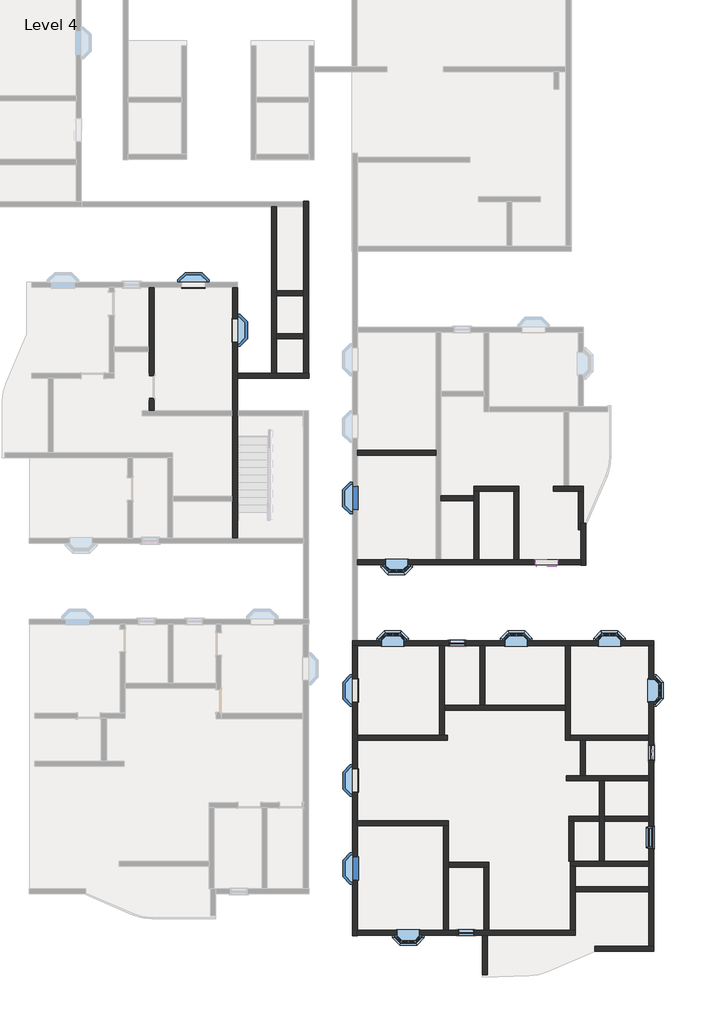
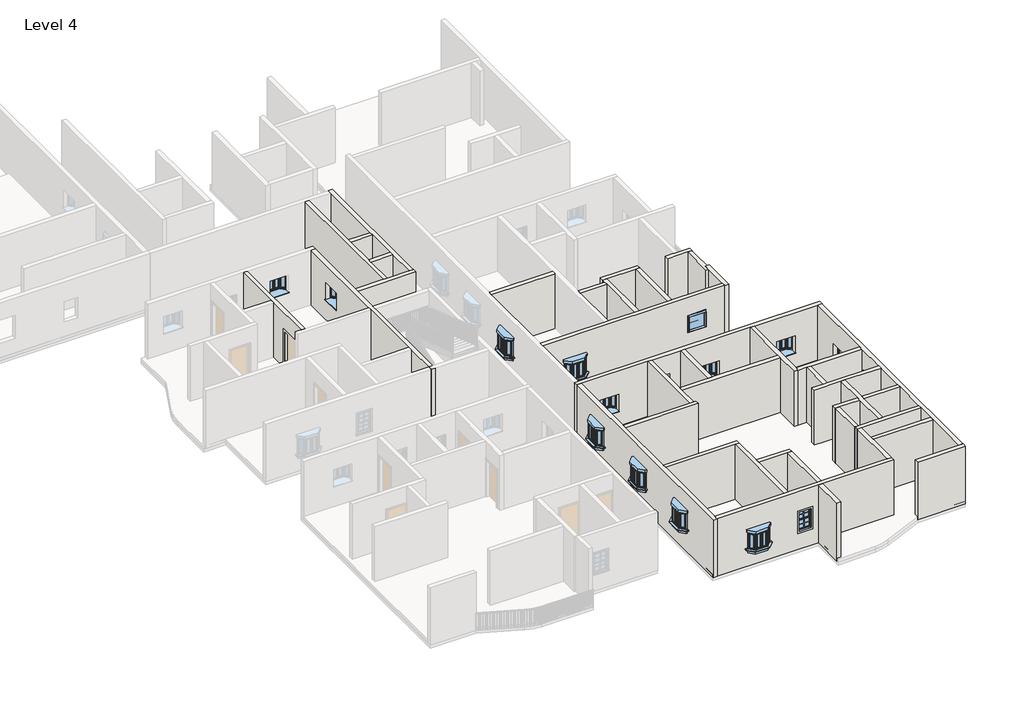
# One storey, part 2 of 14: 40 walls, 17 windows.
# Revit data of these elements (continued)
# Element 46 (IfcWindow, "910x910mm") (continued)
#   Materials on its faces: "Window Frame", "Glass"
# Element 47 (IfcWindow, "910x910mm")
#   Mark = "190"
#   Phase Created = New Construction
#   Materials on its faces: "Window Frame", "Glass"
# Element 48 (IfcWindow, "910x910mm")
#   Mark = "191"
#   Phase Created = New Construction
#   Materials on its faces: "Window Frame", "Glass"
# Element 49 (IfcWindow, "910x910mm")
#   Mark = "192"
#   Phase Created = New Construction
#   Materials on its faces: "Window Frame", "Glass"
# Element 50 (IfcWindow, "910x910mm")
#   Mark = "193"
#   Phase Created = New Construction
#   Materials on its faces: "Window Frame", "Glass"
# Element 51 (IfcWindow, "910x910mm")
#   Mark = "194"
#   Phase Created = New Construction
#   Materials on its faces: "Window Frame", "Glass"
# Element 52 (IfcWindow, "910x910mm")
#   Mark = "195"
#   Phase Created = New Construction
#   Materials on its faces: "Window Frame", "Glass"
# Element 53 (IfcWindow, "Window-Double-Hung : 26\" x 42\"")
#   Mark = "218"
#   Window Inset = 0' - 0"
#   Interior Wall Closure = 0' - 1 1/2"
#   Frame Extension = 0' - 1 1/4"
#   Exterior Wall Closure = 0' - 0 1/2"
#   Interior Trim Visibility = yes
#   Indicator Visibility = yes
#   Exterior Trim Visibility = yes
#   Phase Created = New Construction
#   Materials on its faces: "Wood - Stained", "Glass", "Clad - White"
# Element 54 (IfcWindow, "Window-Double-Hung : 26\" x 42\"")
#   Mark = "219"
#   Window Inset = 0' - 0"
#   Interior Wall Closure = 0' - 1 1/2"
#   Frame Extension = 0' - 1 1/4"
#   Exterior Wall Closure = 0' - 0 1/2"
#   Interior Trim Visibility = yes
#   Indicator Visibility = yes
#   Exterior Trim Visibility = yes
#   Phase Created = New Construction
#   Materials on its faces: "Wood - Stained", "Glass", "Clad - White"
# Element 55 (IfcWindow, "Window-Double-Hung : 26\" x 42\"")
#   Mark = "220"
#   Window Inset = 0' - 0"
#   Interior Wall Closure = 0' - 1 1/2"
#   Frame Extension = 0' - 1 1/4"
#   Exterior Wall Closure = 0' - 0 1/2"
#   Interior Trim Visibility = yes
#   Indicator Visibility = yes
#   Exterior Trim Visibility = yes
#   Phase Created = New Construction
#   Materials on its faces: "Wood - Stained", "Glass", "Clad - White"
# Element 56 (IfcWindow, "Windows_Sgl_w-Glazing_Bars : 910x910mm")
#   Mark = "208"
#   Phase Created = New Construction
#   Materials on its faces: "Window Frame", "Glass"
# Element 57 (IfcWindow, "Windows_Sgl_w-Glazing_Bars : 910x910mm")
#   Mark = "207"
#   Phase Created = New Construction
#   Materials on its faces: "Window Frame", "Glass"
# Materials
#   "Window Frame": colour RGB 249 249 249, transparency 0
#   "Glass": class "Glass", colour RGB 0 128 192, transparency 0.75, Description = "Soda Lime Glass", Cost = 0
#   "Wood - Stained": class "Wood", colour RGB 224 178 126, transparency 0, Cost = 0
#   "Clad - White": class "Wood", colour RGB 242 242 238, transparency 0, Cost = 0
#   "Default Wall": colour RGB 128 128 128, transparency 0, Cost = 0
#   "Door - Frame": colour RGB 118 70 51, transparency 0, Cost = 0
#   "Earth": class "Generic", colour RGB 97 75 62, transparency 0, Description = "Soil", Cost = 0
#   "Carpet (1)": class "Carpet", colour RGB 124 80 67, transparency 0, Description = "Interior finish", Cost = 0
#   "Acoustic Ceiling Tile 24 x 24": class "Generic", colour RGB 232 232 232, transparency 0, Description = "Acoustic Ceiling Tile 24 x 24", Cost = 0
